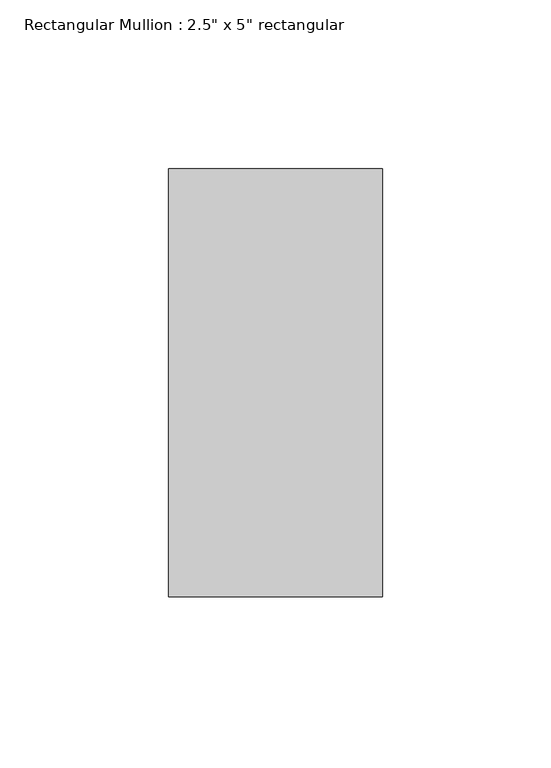
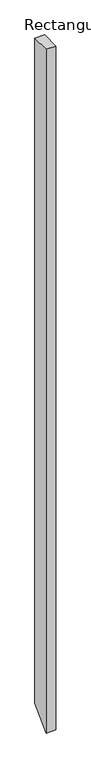
"""IFC4 building model written with IfcOpenShell, lengths in millimetres: member geometry."""

from ifc_helpers import new_model, si_unit, frame, origin, place, context, project, spatial, polyline, outline, extrude, source, transform, mapped, element, save


def member_bdd043b7(model_context):
    return source(origin(), model_context, "Body", "SweptSolid", [
        extrude(outline(polyline([(-63.5, 0.0), (63.5, 0.0), (63.5, -4580.2624252), (-63.5, -4707.2624252), (-63.5, 0.0)])), frame((-63.5, 0.0, 0.0), z_axis=(1.0, 0.0, 0.0), x_axis=(0.0, 1.0, 0.0)), (0.0, 0.0, 1.0), 63.5),
    ])


if __name__ == "__main__":
    model = new_model("IFC4")
    model_context = context("Model", 3, world=origin())
    ifc_project = project(units=[si_unit("LENGTHUNIT", "METRE", prefix="MILLI")], contexts=[model_context])
    site = spatial("IfcSite", under=ifc_project)
    building = spatial("IfcBuilding", under=site)
    placement = place(None, origin())
    member_shape = member_bdd043b7(model_context)
    element("IfcMember", 1, ObjectType="Rectangular Mullion : 2.5\" x 5\" rectangular", at=placement, inside=building, context=model_context, shape_type="MappedRepresentation", body=[
        mapped(member_shape, transform((0.0, 0.0, 0.0), x_axis=(1.0, 0.0, 0.0), y_axis=(0.0, 1.0, 0.0), z_axis=(0.0, 0.0, 1.0))),
    ])
    save(model, "model.ifc")

# Revit data of these elements
# Type "Rectangular Mullion : 2.5\" x 5\" rectangular"
#   built-in parameter 1007304 = 0.416667 (stored number, unit not read)
#   built-in parameter 1007301 = 0.104167 (stored number, unit not read)
#   built-in parameter 1007300 = 0.104167 (stored number, unit not read)
# Element 1 (IfcMember, "Rectangular Mullion : 2.5\" x 5\" rectangular")
#   Materials on its faces: "Aluminum"
# Materials
#   "Aluminum": class "Metal", colour RGB 247 247 247, transparency 0, Description = "Aluminum 6061", Cost = 0
